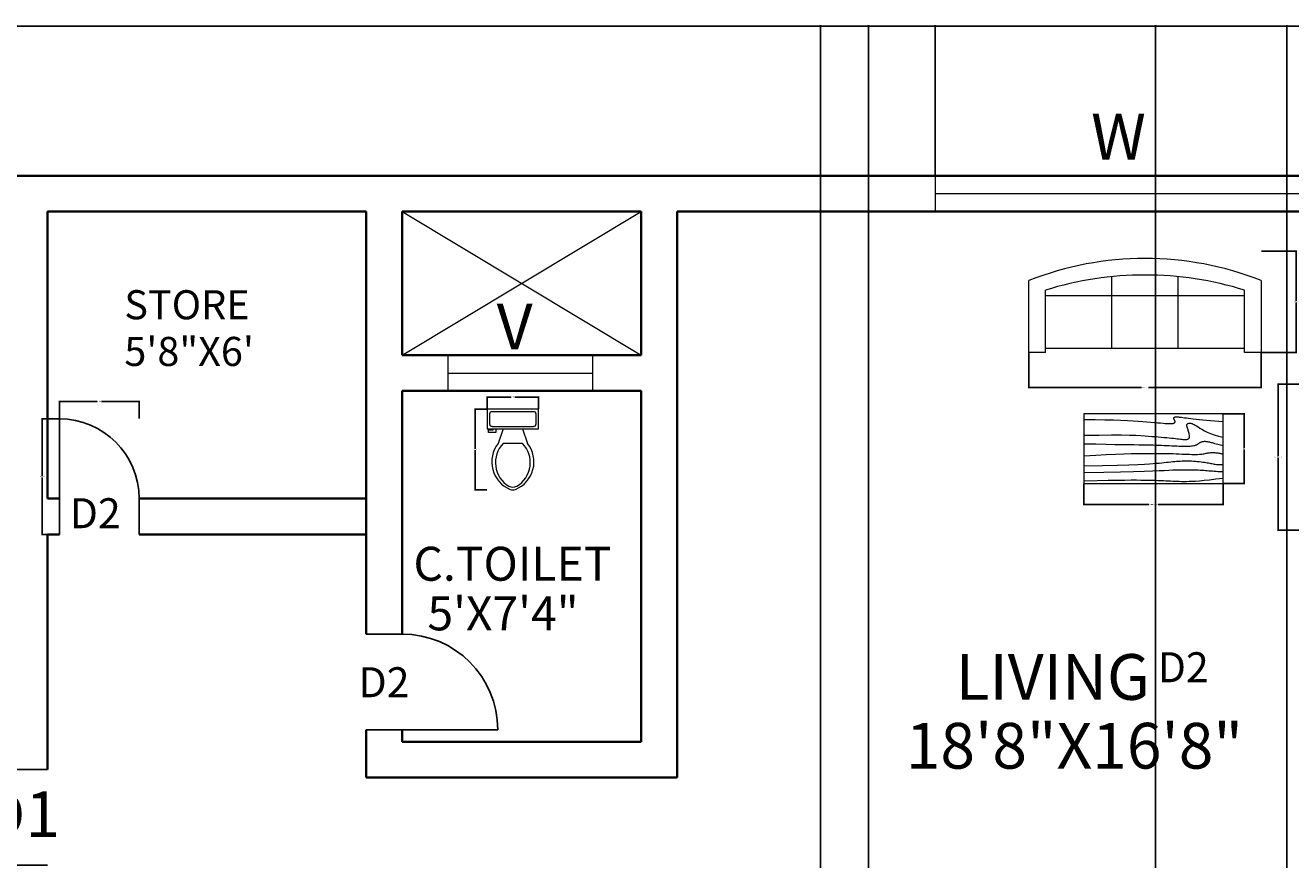
# Model space of a CAD drawing. Units: feet. Extents: x 1889 to 2708, y 1752 to 2375.
# Tile 4 of 5: x 2116 to 2434, y 2166 to 2375. Entities that reach past the tile are written whole.
import ezdxf

# ---------------------------------------------------------------- set-up
doc = ezdxf.new("R2010")
doc.units = ezdxf.units.FT
for name, color, linetype, lineweight in [('A-ANNO-DIMS', 2, 'Continuous', 18), ('A-ANNO-TEXT', 7, 'Continuous', 18), ('A-AREA-IDEN', 7, 'Continuous', 18), ('A-DOOR', 3, 'Continuous', 25), ('A-FLOR-FIXT', 8, 'Continuous', 18), ('A-FLOR-OPEN', 8, 'Continuous', 13), ('A-FURN', 8, 'Continuous', 18), ('A-GLAZ', 4, 'Continuous', 18), ('A-WALL', 7, 'Continuous', 35), ('C-PROP', 7, 'Continuous', 30)]:
    doc.layers.add(name, color=color, linetype=linetype, lineweight=lineweight)
doc.styles.get("Standard").update_dxf_attribs({"font": 'arial.ttf'})
doc.dimstyles.get("Standard").update_dxf_attribs({"dimtxt": 0.18, "dimasz": 0.18, "dimexe": 0.18, "dimexo": 0.0625, "dimgap": 0.09, "dimtad": 0, "dimtih": 1, "dimtoh": 1, "dimdec": 4, "dimzin": 0, "dimdsep": 46, "dimtxsty": 'Standard', "dimcen": 0.09, "dimadec": 0, "dimazin": 0, "dimtfac": 1, "dimtdec": 4, "dimtofl": 0, "dimtmove": 0, "dimatfit": 3, "dimfxl": 1, "dimtolj": 1, "dimtzin": 0, "dimarcsym": 0})

# ---------------------------------------------------------------- blocks, each defined once
blk = doc.blocks.new('Sofa - Roundback 7 ft.')
for p, q in [((-12.00002, -32.4421), (-12.00003, -6.5971)), ((11.99997, -32.4421), (11.99998, -6.5971)), ((-36.000027, -34), (-36.000027, -11.4696)), ((-35.999844, -13.3819), (35.9998, -13.3819)), ((35.99998, -34), (35.99998, -11.4696)), ((-36.000027, -32.4421), (35.99998, -32.4421))]:
    blk.add_line(p, q)
for points in [[(-36.000027, -34), (-42.000027, -34), (-42.000027, -8)], [(41.99998, -8), (41.99998, -34), (35.99998, -34)]]:
    blk.add_lwpolyline(points)
for centre, radius, start, end in [((0, -114.25), 114.25, 68.43141, 111.5686), ((-0.00001, -127.1968), 121.1968, 72.72033, 107.2797)]:
    blk.add_arc(centre, radius, start, end)
blk = doc.blocks.new('Table - Rectangular Woodgrain 60 x 30 in.')
for p, q in [((0, 0), (0, -30)), ((60, 0), (0, 0)), ((60, -30), (60, 0)), ((0, -30), (60, -30))]:
    blk.add_line(p, q)
for points in [[(0, -2.4), (4.8155, -2.418), (9.0302, -2.4688), (12.709, -2.5477), (15.9167, -2.65), (18.7181, -2.7711), (21.1781, -2.9063), (23.3616, -3.0508), (25.3333, -3.2), (27.1477, -3.3495), (28.8172, -3.4958), (30.3437, -3.636), (31.7291, -3.7667), (32.9756, -3.8849), (34.0849, -3.9875), (35.059, -4.0714), (35.9, -4.1334), (36.6114, -4.1711), (37.2041, -4.1854), (37.6906, -4.1779), (38.0833, -4.15), (38.3948, -4.1034), (38.6375, -4.0396), (38.8239, -3.9602), (38.9666, -3.8667), (39.0764, -3.7608), (39.1573, -3.6448), (39.2116, -3.521), (39.2416, -3.3917), (39.2498, -3.2593), (39.2385, -3.1261), (39.21, -2.9944), (39.1666, -2.8667), (39.111, -2.7447), (39.0468, -2.6281), (38.978, -2.5163), (38.9083, -2.4083), (38.8418, -2.3035), (38.7823, -2.201), (38.7337, -2.1001), (38.7, -2), (38.6844, -1.9003), (38.6875, -1.8021), (38.7094, -1.707), (38.75, -1.6167), (38.8094, -1.5326), (38.8875, -1.4563), (38.9844, -1.3893), (39.1, -1.3333), (39.2351, -1.2896), (39.3937, -1.2583), (39.5804, -1.2396), (39.8, -1.2333), (40.057, -1.2396), (40.3562, -1.2583), (40.7023, -1.2896), (41.1, -1.3333), (41.5547, -1.3895), (42.0755, -1.4573), (42.6721, -1.5361), (43.3542, -1.625), (44.1316, -1.7233), (45.014, -1.8302), (46.0114, -1.9449), (47.1333, -2.0667), (48.3862, -2.1947), (49.7625, -2.3281), (51.2513, -2.4663), (52.8416, -2.6083), (54.5226, -2.7535), (56.2833, -2.9011), (58.1127, -3.0501), (60, -3.2)], [(0, -9.2), (6.5759, -9.0858), (11.9385, -9.0365), (16.2527, -9.0418), (19.6833, -9.0917), (22.3952, -9.1759), (24.5531, -9.2844), (26.322, -9.4069), (27.8666, -9.5333), (29.3241, -9.6553), (30.7203, -9.7719), (32.0532, -9.8837), (33.3208, -9.9917), (34.5213, -10.0965), (35.6526, -10.199), (36.7128, -10.2999), (37.7, -10.4), (38.6129, -10.4996), (39.4531, -10.5969), (40.223, -10.6895), (40.925, -10.775), (41.5613, -10.8512), (42.1344, -10.9156), (42.6465, -10.966), (43.1, -11), (43.4976, -11.0158), (43.8437, -11.0136), (44.143, -10.9942), (44.4, -10.9583), (44.6195, -10.9069), (44.8062, -10.8406), (44.9648, -10.7603), (45.1, -10.6667), (45.2155, -10.5598), (45.3114, -10.4365), (45.3871, -10.2929), (45.4416, -10.125), (45.4743, -9.929), (45.4844, -9.7011), (45.4709, -9.4371), (45.4333, -9.1333), (45.3716, -8.7883), (45.2896, -8.4104), (45.1919, -8.0107), (45.0833, -7.6), (44.9685, -7.1893), (44.8521, -6.7896), (44.7388, -6.4117), (44.6333, -6.0667), (44.54, -5.7628), (44.4614, -5.4979), (44.4001, -5.2675), (44.3583, -5.0667), (44.3384, -4.8909), (44.3427, -4.7354), (44.3736, -4.5956), (44.4333, -4.4667), (44.5236, -4.3453), (44.6427, -4.2333), (44.7884, -4.1339), (44.9583, -4.05), (45.1501, -3.9849), (45.3614, -3.9417), (45.59, -3.9234), (45.8333, -3.9333), (46.0915, -3.9749), (46.3734, -4.0531), (46.6906, -4.1736), (47.0542, -4.3417), (47.4756, -4.5629), (47.9661, -4.8427), (48.5372, -5.1866), (49.2, -5.6), (49.9676, -6.0844), (50.8594, -6.625), (51.8965, -7.2031), (53.1, -7.8), (54.491, -8.3969), (56.0906, -8.975), (57.9199, -9.5156), (60, -10)], [(0, -12.8), (5.1847, -12.9322), (9.6213, -13.0323), (13.3963, -13.1059), (16.5958, -13.1583), (19.3063, -13.1952), (21.614, -13.2219), (23.6054, -13.2439), (25.3666, -13.2667), (26.9728, -13.2947), (28.4531, -13.3281), (29.8256, -13.3663), (31.1083, -13.4083), (32.3191, -13.4535), (33.476, -13.501), (34.597, -13.5501), (35.7, -13.6), (36.7984, -13.6497), (37.8875, -13.6979), (38.9578, -13.743), (40, -13.7833), (41.0047, -13.8174), (41.9625, -13.8438), (42.864, -13.8607), (43.7, -13.8667), (44.4631, -13.8604), (45.1552, -13.8417), (45.7801, -13.8104), (46.3416, -13.7667), (46.8439, -13.7104), (47.2906, -13.6417), (47.6858, -13.5604), (48.0333, -13.4667), (48.3375, -13.3608), (48.6042, -13.2448), (48.8396, -13.121), (49.05, -12.9917), (49.2417, -12.8593), (49.4208, -12.7261), (49.5937, -12.5944), (49.7667, -12.4667), (49.9452, -12.3451), (50.1323, -12.2313), (50.3303, -12.1268), (50.5416, -12.0333), (50.7686, -11.9524), (51.0135, -11.8854), (51.2788, -11.8341), (51.5666, -11.8), (51.8785, -11.7843), (52.2116, -11.7865), (52.562, -11.8059), (52.926, -11.8417), (53.2998, -11.8931), (53.6795, -11.9594), (54.0614, -12.0397), (54.4416, -12.1333), (54.8223, -12.2401), (55.2293, -12.3625), (55.6942, -12.5037), (56.2489, -12.6667), (56.9251, -12.8547), (57.7545, -13.0708), (58.7689, -13.3182), (60, -13.6)], [(0, -18), (5.124, -17.7273), (9.6609, -17.5057), (13.6705, -17.3303), (17.2125, -17.1958), (20.3467, -17.0973), (23.1328, -17.0297), (25.6307, -16.9878), (27.9, -16.9667), (29.9928, -16.9617), (31.9302, -16.9703), (33.7254, -16.9907), (35.3917, -17.0208), (36.9423, -17.0588), (38.3906, -17.1026), (39.7499, -17.1503), (41.0333, -17.2), (42.2519, -17.2496), (43.4073, -17.2969), (44.4986, -17.3395), (45.525, -17.375), (46.4858, -17.4012), (47.3802, -17.4156), (48.2074, -17.416), (48.9667, -17.4), (49.6583, -17.3662), (50.2872, -17.3167), (50.8595, -17.2547), (51.3812, -17.1833), (51.8584, -17.1057), (52.2971, -17.025), (52.7034, -16.9443), (53.0833, -16.8667), (53.443, -16.7951), (53.789, -16.7313), (54.128, -16.6768), (54.4666, -16.6334), (54.8115, -16.6024), (55.1693, -16.5854), (55.5465, -16.5841), (55.95, -16.6), (56.3828, -16.6337), (56.8346, -16.6823), (57.2915, -16.7418), (57.7396, -16.8084), (58.165, -16.878), (58.5539, -16.9469), (58.8924, -17.0111), (59.1666, -17.0667), (59.3679, -17.1107), (59.5078, -17.1438), (59.6032, -17.1675), (59.6708, -17.1833), (59.7275, -17.193), (59.7901, -17.1979), (59.8753, -17.1998), (60, -17.2)], [(0, -22.4), (8.0098, -22.2501), (14.4094, -22.1011), (19.4168, -21.9535), (23.25, -21.8083), (26.1269, -21.6663), (28.2656, -21.5281), (29.884, -21.3947), (31.2, -21.2667), (32.3967, -21.1448), (33.5172, -21.0292), (34.5697, -20.9198), (35.5625, -20.8167), (36.5037, -20.7198), (37.4015, -20.6292), (38.2642, -20.5448), (39.1, -20.4667), (39.9164, -20.3951), (40.7187, -20.3313), (41.5117, -20.2768), (42.3, -20.2333), (43.0883, -20.2024), (43.8812, -20.1854), (44.6836, -20.1841), (45.5, -20.2), (46.3328, -20.234), (47.1747, -20.2844), (48.0163, -20.3488), (48.8479, -20.425), (49.66, -20.5106), (50.4429, -20.6031), (51.1872, -20.7004), (51.8833, -20.8), (52.5246, -20.8999), (53.1166, -20.9995), (53.6681, -21.0983), (54.1875, -21.1958), (54.6834, -21.2919), (55.1646, -21.3859), (55.6394, -21.4777), (56.1167, -21.5667), (56.6028, -21.6515), (57.0961, -21.7266), (57.5929, -21.7852), (58.0896, -21.8208), (58.5823, -21.8268), (59.0674, -21.7964), (59.5412, -21.723), (60, -21.6)], [(0, -25.2), (8.6355, -25.0504), (15.7026, -24.9031), (21.4049, -24.7606), (25.9458, -24.625), (29.529, -24.4988), (32.3578, -24.3844), (34.6359, -24.284), (36.5667, -24.2), (38.3213, -24.1341), (39.9417, -24.0854), (41.437, -24.0523), (42.8167, -24.0333), (44.0901, -24.0268), (45.2667, -24.0313), (46.3557, -24.0451), (47.3667, -24.0667), (48.309, -24.0947), (49.1928, -24.1287), (50.0284, -24.168), (50.826, -24.2125), (51.5959, -24.2617), (52.3483, -24.3151), (53.0935, -24.3725), (53.8417, -24.4334), (54.6009, -24.497), (55.3699, -24.561), (56.1454, -24.6226), (56.9239, -24.6792), (57.7021, -24.7279), (58.4764, -24.7662), (59.2435, -24.7911), (60, -24.8)], [(0, -28.8), (5.6867, -28.6681), (10.45, -28.5698), (14.407, -28.5012), (17.675, -28.4584), (20.3711, -28.4374), (22.6125, -28.4344), (24.5164, -28.4455), (26.2, -28.4667), (27.762, -28.4947), (29.2276, -28.5281), (30.6033, -28.5663), (31.8958, -28.6084), (33.1118, -28.6535), (34.2578, -28.7011), (35.3405, -28.7501), (36.3666, -28.8), (37.3443, -28.8497), (38.288, -28.8974), (39.2137, -28.9412), (40.1375, -28.9792), (41.0753, -29.0093), (42.0432, -29.0297), (43.0572, -29.0384), (44.1333, -29.0333), (45.2936, -29.0114), (46.5843, -28.9641), (48.0579, -28.8816), (49.7666, -28.7542), (51.7629, -28.5721), (54.0989, -28.3255), (56.8272, -28.0048), (60, -27.6)]]:
    blk.add_lwpolyline(points)
blk = doc.blocks.new('Toilet - top')
for p, q in [((9.5, -6), (9.5, -2)), ((-10, -8.5), (-8, -8.5)), ((-10, -9.5), (-10, -8.5)), ((-7, -9.5), (-10, -9.5)), ((-8, -8.5), (-8, -8)), ((-7, -8), (-7, -9.5)), ((-4, -8), (-6, -14)), ((4, -8), (6, -14)), ((4, -14), (-4, -14))]:
    blk.add_line(p, q)
blk.add_lwpolyline([(10.5, -8), (10.5, 0), (-10.5, 0), (-10.5, -8)], close=True)
for points in [[(-9.5, -2), (-9.5, -6)], [(8.5, -1), (-8.5, -1)], [(-8.5, -7), (8.5, -7)]]:
    blk.add_lwpolyline(points)
for centre, radius, start, end in [((-8.62, -1.88), 0.884, 81.8699, 188.1301), ((8.62, -1.88), 0.884, 351.8699, 98.1301), ((-8.62, -6.12), 0.884, 171.8699, 278.1301), ((8.62, -6.12), 0.884, 261.8699, 8.1301), ((3.52, -21.58), 12.17, 141.4691, 247.9714), ((4.2, -21.82), 11.33, 136.3677, 238.9468), ((-3.52, -21.58), 12.17, 292.0284, 38.5307), ((-4.2, -21.82), 11.33, 301.053, 43.6321), ((0, -27.88), 4, 245.7318, 294.2682), ((0, -29), 4, 254.8605, 285.1395)]:
    blk.add_arc(centre, radius, start, end)
blk = doc.blocks.new('DOOR-SWING-24')
for p, q in [((9, 24), (0, 24)), ((33, 0), (0, 0))]:
    blk.add_line(p, q)
blk.add_arc((9, 0), 24, 0, 90)
blk = doc.blocks.new('DOOR-SWING-20')
for p, q in [((0, 29), (0, 0)), ((20, 9), (20, 0))]:
    blk.add_line(p, q)
blk.add_arc((0, 9), 20, 0, 90)
blk = doc.blocks.new('*D15')
at = {"layer": 'A-ANNO-DIMS', "color": 0, "lineweight": -2, "transparency": 16777216}
for p, q in [((2124.8, 2276.6), (2120.33, 2276.6)), ((2120.51, 2276.42), (2120.51, 2262.28)), ((2120.51, 2247.78), (2120.51, 2261.92)), ((2124.8, 2247.6), (2120.33, 2247.6))]:
    blk.add_line(p, q, dxfattribs=at)
at = {"layer": 'A-ANNO-DIMS', "color": 0, "transparency": 16777216}
for points in [[(2120.48, 2276.42), (2120.54, 2276.42), (2120.51, 2276.6)], [(2120.48, 2247.78), (2120.54, 2247.78), (2120.51, 2247.6)]]:
    blk.add_solid(points, dxfattribs=at)
at = {"layer": 'Defpoints', "color": 0, "transparency": 16777216}
for p in [(2120.51, 2276.6), (2124.86, 2276.6), (2124.86, 2247.6)]:
    blk.add_point(p, dxfattribs=at)
at = {"layer": 'A-ANNO-DIMS', "color": 0, "transparency": 16777216, "insert": (2120.51, 2262.1), "char_height": 0.18, "attachment_point": 5}
blk.add_mtext('\\A1;DOOR 29 TYP.', dxfattribs=at)
blk = doc.blocks.new('*D16')
at = {"layer": 'A-ANNO-DIMS', "color": 0, "lineweight": -2, "transparency": 16777216}
for p, q in [((2124.86, 2276.66), (2124.86, 2281.13)), ((2125.04, 2280.95), (2134.33, 2280.95)), ((2144.68, 2280.95), (2135.39, 2280.95)), ((2144.86, 2276.66), (2144.86, 2281.13))]:
    blk.add_line(p, q, dxfattribs=at)
at = {"layer": 'A-ANNO-DIMS', "color": 0, "transparency": 16777216}
for points in [[(2125.04, 2280.98), (2125.04, 2280.92), (2124.86, 2280.95)], [(2144.68, 2280.98), (2144.68, 2280.92), (2144.86, 2280.95)]]:
    blk.add_solid(points, dxfattribs=at)
at = {"layer": 'Defpoints', "color": 0, "transparency": 16777216}
for p in [(2144.86, 2280.95), (2124.86, 2276.6), (2144.86, 2276.6)]:
    blk.add_point(p, dxfattribs=at)
at = {"layer": 'A-ANNO-DIMS', "color": 0, "transparency": 16777216, "insert": (2134.86, 2280.95), "char_height": 0.18, "attachment_point": 5}
blk.add_mtext('\\A1;20 TYP.', dxfattribs=at)
blk = doc.blocks.new('*D17')
at = {"layer": 'A-ANNO-DIMS', "color": 0, "lineweight": -2, "transparency": 16777216}
for p, q in [((2232.14, 2279.01), (2228.98, 2279.01)), ((2229.16, 2278.83), (2229.16, 2269.07)), ((2229.16, 2258.94), (2229.16, 2268.7)), ((2232.14, 2258.76), (2228.98, 2258.76))]:
    blk.add_line(p, q, dxfattribs=at)
at = {"layer": 'A-ANNO-DIMS', "color": 0, "transparency": 16777216}
for points in [[(2229.13, 2278.83), (2229.19, 2278.83), (2229.16, 2279.01)], [(2229.13, 2258.94), (2229.19, 2258.94), (2229.16, 2258.76)]]:
    blk.add_solid(points, dxfattribs=at)
at = {"layer": 'Defpoints', "color": 0, "transparency": 16777216}
for p in [(2229.16, 2279.01), (2232.2, 2279.01), (2232.2, 2258.76)]:
    blk.add_point(p, dxfattribs=at)
at = {"layer": 'A-ANNO-DIMS', "color": 0, "transparency": 16777216, "insert": (2229.16, 2268.88), "char_height": 0.18, "attachment_point": 5}
blk.add_mtext('\\A1;WC 20 TYP.', dxfattribs=at)
blk = doc.blocks.new('*D18')
at = {"layer": 'A-ANNO-DIMS', "color": 0, "lineweight": -2, "transparency": 16777216}
for p, q in [((2232.2, 2279.07), (2232.2, 2282.22)), ((2232.38, 2282.04), (2238.11, 2282.04)), ((2244.88, 2282.04), (2239.15, 2282.04)), ((2245.06, 2279.07), (2245.06, 2282.22))]:
    blk.add_line(p, q, dxfattribs=at)
at = {"layer": 'A-ANNO-DIMS', "color": 0, "transparency": 16777216}
for points in [[(2232.38, 2282.07), (2232.38, 2282.01), (2232.2, 2282.04)], [(2244.88, 2282.07), (2244.88, 2282.01), (2245.06, 2282.04)]]:
    blk.add_solid(points, dxfattribs=at)
at = {"layer": 'Defpoints', "color": 0, "transparency": 16777216}
for p in [(2245.06, 2282.04), (2232.2, 2279.01), (2245.06, 2279.01)]:
    blk.add_point(p, dxfattribs=at)
at = {"layer": 'A-ANNO-DIMS', "color": 0, "transparency": 16777216, "insert": (2238.63, 2282.04), "char_height": 0.18, "attachment_point": 5}
blk.add_mtext('\\A1;13 TYP.', dxfattribs=at)
blk = doc.blocks.new('*D23')
at = {"layer": 'A-ANNO-DIMS', "color": 0, "lineweight": -2, "transparency": 16777216}
for p, q in [((2368.1, 2293.18), (2368.1, 2284.32)), ((2426.4, 2293.18), (2426.4, 2284.32)), ((2368.28, 2284.5), (2396.35, 2284.5)), ((2426.22, 2284.5), (2398.16, 2284.5))]:
    blk.add_line(p, q, dxfattribs=at)
at = {"layer": 'A-ANNO-DIMS', "color": 0, "transparency": 16777216}
for points in [[(2368.28, 2284.53), (2368.28, 2284.47), (2368.1, 2284.5)], [(2426.22, 2284.53), (2426.22, 2284.47), (2426.4, 2284.5)]]:
    blk.add_solid(points, dxfattribs=at)
at = {"layer": 'Defpoints', "color": 0, "transparency": 16777216}
for p in [(2368.1, 2293.24), (2426.4, 2293.24), (2426.4, 2284.5)]:
    blk.add_point(p, dxfattribs=at)
at = {"layer": 'A-ANNO-DIMS', "color": 0, "transparency": 16777216, "insert": (2397.25, 2284.5), "char_height": 0.18, "attachment_point": 5}
blk.add_mtext('\\A1;SOFA 58 TYP.', dxfattribs=at)
blk = doc.blocks.new('*D24')
at = {"layer": 'A-ANNO-DIMS', "color": 0, "lineweight": -2, "transparency": 16777216}
for p, q in [((2426.47, 2318.69), (2435.33, 2318.69)), ((2435.15, 2318.51), (2435.15, 2306.15)), ((2435.15, 2293.42), (2435.15, 2305.78)), ((2426.47, 2293.24), (2435.33, 2293.24))]:
    blk.add_line(p, q, dxfattribs=at)
at = {"layer": 'A-ANNO-DIMS', "color": 0, "transparency": 16777216}
for points in [[(2435.12, 2318.51), (2435.18, 2318.51), (2435.15, 2318.69)], [(2435.12, 2293.42), (2435.18, 2293.42), (2435.15, 2293.24)]]:
    blk.add_solid(points, dxfattribs=at)
at = {"layer": 'Defpoints', "color": 0, "transparency": 16777216}
for p in [(2426.4, 2318.69), (2435.15, 2318.69), (2426.4, 2293.24)]:
    blk.add_point(p, dxfattribs=at)
at = {"layer": 'A-ANNO-DIMS', "color": 0, "transparency": 16777216, "insert": (2435.15, 2305.97), "char_height": 0.18, "attachment_point": 5}
blk.add_mtext('\\A1;25 TYP.', dxfattribs=at)
blk = doc.blocks.new('*D25')
at = {"layer": 'A-ANNO-DIMS', "color": 0, "lineweight": -2, "transparency": 16777216}
for p, q in [((2436.07, 2285.32), (2430.47, 2285.32)), ((2430.65, 2285.14), (2430.65, 2267.2)), ((2430.65, 2248.89), (2430.65, 2266.83)), ((2436.07, 2248.71), (2430.47, 2248.71))]:
    blk.add_line(p, q, dxfattribs=at)
at = {"layer": 'A-ANNO-DIMS', "color": 0, "transparency": 16777216}
for points in [[(2430.62, 2285.14), (2430.68, 2285.14), (2430.65, 2285.32)], [(2430.62, 2248.89), (2430.68, 2248.89), (2430.65, 2248.71)]]:
    blk.add_solid(points, dxfattribs=at)
at = {"layer": 'Defpoints', "color": 0, "transparency": 16777216}
for p in [(2436.14, 2285.32), (2430.65, 2248.71), (2436.14, 2248.71)]:
    blk.add_point(p, dxfattribs=at)
at = {"layer": 'A-ANNO-DIMS', "color": 0, "transparency": 16777216, "insert": (2430.65, 2267.01), "char_height": 0.18, "attachment_point": 5}
blk.add_mtext('\\A1;LOVESEAT 37 TYP.', dxfattribs=at)
blk = doc.blocks.new('*D29')
at = {"layer": 'A-ANNO-DIMS', "color": 0, "lineweight": -2, "transparency": 16777216}
for p, q in [((2381.91, 2260.29), (2381.91, 2254.93)), ((2416.86, 2260.29), (2416.86, 2254.93)), ((2382.09, 2255.11), (2398.19, 2255.11)), ((2416.68, 2255.11), (2400.58, 2255.11))]:
    blk.add_line(p, q, dxfattribs=at)
at = {"layer": 'A-ANNO-DIMS', "color": 0, "transparency": 16777216}
for points in [[(2382.09, 2255.14), (2382.09, 2255.08), (2381.91, 2255.11)], [(2416.68, 2255.14), (2416.68, 2255.08), (2416.86, 2255.11)]]:
    blk.add_solid(points, dxfattribs=at)
at = {"layer": 'Defpoints', "color": 0, "transparency": 16777216}
for p in [(2381.91, 2260.35), (2416.86, 2260.35), (2416.86, 2255.11)]:
    blk.add_point(p, dxfattribs=at)
at = {"layer": 'A-ANNO-DIMS', "color": 0, "transparency": 16777216, "insert": (2399.38, 2255.11), "char_height": 0.18, "attachment_point": 5}
blk.add_mtext('\\A1;COFFEE TABLE 35', dxfattribs=at)
blk = doc.blocks.new('*D30')
at = {"layer": 'A-ANNO-DIMS', "color": 0, "lineweight": -2, "transparency": 16777216}
for p, q in [((2416.93, 2277.83), (2422.29, 2277.83)), ((2422.11, 2277.65), (2422.11, 2269.27)), ((2422.11, 2260.53), (2422.11, 2268.91)), ((2416.93, 2260.35), (2422.29, 2260.35))]:
    blk.add_line(p, q, dxfattribs=at)
at = {"layer": 'A-ANNO-DIMS', "color": 0, "transparency": 16777216}
for points in [[(2422.08, 2277.65), (2422.14, 2277.65), (2422.11, 2277.83)], [(2422.08, 2260.53), (2422.14, 2260.53), (2422.11, 2260.35)]]:
    blk.add_solid(points, dxfattribs=at)
at = {"layer": 'Defpoints', "color": 0, "transparency": 16777216}
for p in [(2416.86, 2277.83), (2422.11, 2277.83), (2416.86, 2260.35)]:
    blk.add_point(p, dxfattribs=at)
at = {"layer": 'A-ANNO-DIMS', "color": 0, "transparency": 16777216, "insert": (2422.11, 2269.09), "char_height": 0.18, "attachment_point": 5}
blk.add_mtext('\\A1;17', dxfattribs=at)
blk = doc.blocks.new('*D38')
at = {"layer": 'A-ANNO-DIMS', "color": 0, "lineweight": -2, "transparency": 16777216}
for p, q in [((2082.41, 2337.66), (2082.41, 2375.33)), ((2082.59, 2375.15), (2213.05, 2375.15)), ((2344.45, 2375.15), (2213.98, 2375.15)), ((2344.63, 2337.66), (2344.63, 2375.33))]:
    blk.add_line(p, q, dxfattribs=at)
at = {"layer": 'A-ANNO-DIMS', "color": 0, "transparency": 16777216}
for points in [[(2082.59, 2375.18), (2082.59, 2375.12), (2082.41, 2375.15)], [(2344.45, 2375.18), (2344.45, 2375.12), (2344.63, 2375.15)]]:
    blk.add_solid(points, dxfattribs=at)
at = {"layer": 'Defpoints', "color": 0, "transparency": 16777216}
for p in [(2344.63, 2375.15), (2082.41, 2337.6), (2344.63, 2337.6)]:
    blk.add_point(p, dxfattribs=at)
at = {"layer": 'A-ANNO-DIMS', "color": 0, "transparency": 16777216, "insert": (2213.52, 2375.15), "char_height": 0.18, "attachment_point": 5}
blk.add_mtext('\\A1;262.23', dxfattribs=at)
blk = doc.blocks.new('*D39')
at = {"layer": 'A-ANNO-DIMS', "color": 0, "lineweight": -2, "transparency": 16777216}
for p, q in [((2344.63, 2337.66), (2344.63, 2375.33)), ((2344.81, 2375.15), (2395.36, 2375.15)), ((2446.46, 2375.15), (2395.92, 2375.15)), ((2446.64, 2337.66), (2446.64, 2375.33))]:
    blk.add_line(p, q, dxfattribs=at)
at = {"layer": 'A-ANNO-DIMS', "color": 0, "transparency": 16777216}
for points in [[(2344.81, 2375.18), (2344.81, 2375.12), (2344.63, 2375.15)], [(2446.46, 2375.18), (2446.46, 2375.12), (2446.64, 2375.15)]]:
    blk.add_solid(points, dxfattribs=at)
at = {"layer": 'Defpoints', "color": 0, "transparency": 16777216}
for p in [(2446.64, 2375.15), (2344.63, 2337.6), (2446.64, 2337.6)]:
    blk.add_point(p, dxfattribs=at)
at = {"layer": 'A-ANNO-DIMS', "color": 0, "transparency": 16777216, "insert": (2395.64, 2375.15), "char_height": 0.18, "attachment_point": 5}
blk.add_mtext('\\A1;102', dxfattribs=at)
blk = doc.blocks.new('*D48')
at = {"layer": 'A-ANNO-DIMS', "color": 0, "lineweight": -2, "transparency": 16777216}
for p, q in [((1983.86, 1820.66), (1983.86, 2375.33)), ((1984.04, 2375.15), (2208.07, 2375.15)), ((2432.68, 2375.15), (2208.66, 2375.15)), ((2432.86, 1820.66), (2432.86, 2375.33))]:
    blk.add_line(p, q, dxfattribs=at)
at = {"layer": 'A-ANNO-DIMS', "color": 0, "transparency": 16777216}
for points in [[(1984.04, 2375.18), (1984.04, 2375.12), (1983.86, 2375.15)], [(2432.68, 2375.18), (2432.68, 2375.12), (2432.86, 2375.15)]]:
    blk.add_solid(points, dxfattribs=at)
at = {"layer": 'Defpoints', "color": 0, "transparency": 16777216}
for p in [(2432.86, 2375.15), (1983.86, 1820.6), (2432.86, 1820.6)]:
    blk.add_point(p, dxfattribs=at)
at = {"layer": 'A-ANNO-DIMS', "color": 0, "transparency": 16777216, "insert": (2208.36, 2375.15), "char_height": 0.18, "attachment_point": 5}
blk.add_mtext('\\A1;449', dxfattribs=at)
blk = doc.blocks.new('*D61')
at = {"layer": 'A-ANNO-DIMS', "color": 0, "lineweight": -2, "transparency": 16777216}
for p, q in [((2315.86, 1909.16), (2315.86, 2375.33)), ((2316.04, 2375.15), (2321.65, 2375.15)), ((2327.68, 2375.15), (2322.07, 2375.15)), ((2327.86, 1913.66), (2327.86, 2375.33))]:
    blk.add_line(p, q, dxfattribs=at)
at = {"layer": 'A-ANNO-DIMS', "color": 0, "transparency": 16777216}
for points in [[(2316.04, 2375.18), (2316.04, 2375.12), (2315.86, 2375.15)], [(2327.68, 2375.18), (2327.68, 2375.12), (2327.86, 2375.15)]]:
    blk.add_solid(points, dxfattribs=at)
at = {"layer": 'Defpoints', "color": 0, "transparency": 16777216}
for p in [(2327.86, 2375.15), (2327.86, 1913.6), (2315.86, 1909.1)]:
    blk.add_point(p, dxfattribs=at)
at = {"layer": 'A-ANNO-DIMS', "color": 0, "transparency": 16777216, "insert": (2321.86, 2375.15), "char_height": 0.18, "attachment_point": 5}
blk.add_mtext('\\A1;12', dxfattribs=at)
blk = doc.blocks.new('*D64')
at = {"layer": 'A-ANNO-DIMS', "color": 0, "lineweight": -2, "transparency": 16777216}
for p, q in [((2327.86, 2011.66), (2327.86, 2375.33)), ((2328.04, 2375.15), (2363.65, 2375.15)), ((2399.68, 2375.15), (2364.08, 2375.15)), ((2399.86, 2011.66), (2399.86, 2375.33))]:
    blk.add_line(p, q, dxfattribs=at)
at = {"layer": 'A-ANNO-DIMS', "color": 0, "transparency": 16777216}
for points in [[(2328.04, 2375.18), (2328.04, 2375.12), (2327.86, 2375.15)], [(2399.68, 2375.18), (2399.68, 2375.12), (2399.86, 2375.15)]]:
    blk.add_solid(points, dxfattribs=at)
at = {"layer": 'Defpoints', "color": 0, "transparency": 16777216}
for p in [(2399.86, 2375.15), (2327.86, 2011.6), (2399.86, 2011.6)]:
    blk.add_point(p, dxfattribs=at)
at = {"layer": 'A-ANNO-DIMS', "color": 0, "transparency": 16777216, "insert": (2363.86, 2375.15), "char_height": 0.18, "attachment_point": 5}
blk.add_mtext('\\A1;72', dxfattribs=at)

msp = doc.modelspace()

# ---------------------------------------------------------------- linework, layer by layer
at = {"layer": 'A-FLOR-OPEN'}
for p, q in [((2210.8644, 2328.5988), (2270.8644, 2292.5988)), ((2210.8644, 2292.5988), (2270.8644, 2328.5988))]:
    msp.add_line(p, q, dxfattribs=at)
at = {"layer": 'A-GLAZ'}
for p, q in [((2344.6329, 2337.5988), (2344.6329, 2328.5988)), ((2344.6329, 2333.0988), (2446.6414, 2333.0988)), ((2222.3553, 2292.5988), (2222.3553, 2283.5988)), ((2258.6501, 2292.5988), (2258.6501, 2283.5988)), ((2222.3553, 2288.0988), (2258.6501, 2288.0988))]:
    msp.add_line(p, q, dxfattribs=at)
at = {"layer": 'A-WALL'}
for p, q in [((1992.8644, 2337.5988), (2669.8644, 2337.5988)), ((2121.8644, 2337.5988), (2201.8644, 2337.5988)), ((2210.8644, 2337.5988), (2270.8644, 2337.5988)), ((2279.8644, 2337.5988), (2503.8644, 2337.5988)), ((2121.8644, 2328.5988), (2121.8644, 2256.5988)), ((2121.8644, 2328.5988), (2201.8644, 2328.5988)), ((2201.8644, 2328.5988), (2201.8644, 2256.5988)), ((2210.8644, 2328.5988), (2210.8644, 2292.5988)), ((2210.8644, 2328.5988), (2270.8644, 2328.5988)), ((2270.8644, 2328.5988), (2270.8644, 2292.5988)), ((2279.8644, 2328.5988), (2279.8644, 2186.5988)), ((2279.8644, 2328.5988), (2503.8644, 2328.5988)), ((2270.8644, 2292.5988), (2210.8644, 2292.5988)), ((2270.8644, 2283.5988), (2210.8644, 2283.5988)), ((2210.8644, 2283.5988), (2210.8644, 2256.5988)), ((2270.8644, 2283.5988), (2270.8644, 2195.5988)), ((2279.8644, 2283.5988), (2279.8644, 2195.5988)), ((2124.8644, 2256.5988), (2121.8644, 2256.5988)), ((2201.8644, 2256.5988), (2144.8644, 2256.5988)), ((2201.8644, 2222.5988), (2201.8644, 2256.5988)), ((2210.8644, 2222.5988), (2210.8644, 2256.5988)), ((2121.8644, 2247.5988), (2121.8644, 2188.5988)), ((2124.8644, 2247.5988), (2121.8644, 2247.5988)), ((2201.8644, 2247.5988), (2144.8644, 2247.5988)), ((2201.8644, 2186.5988), (2201.8644, 2198.5988)), ((2210.8644, 2195.5988), (2210.8644, 2198.5988)), ((2270.8644, 2195.5988), (2210.8644, 2195.5988)), ((2279.8644, 2186.5988), (2279.8644, 2195.5988)), ((2121.8644, 2188.5988), (2121.8644, 2191.5988)), ((2279.8644, 2186.5988), (2201.8644, 2186.5988))]:
    msp.add_line(p, q, dxfattribs=at)
at = {"layer": 'C-PROP'}
msp.add_line((1926.8644, 2337.5988), (2669.8644, 2337.5988), dxfattribs=at)

# ---------------------------------------------------------------- block references
at = {"layer": 'A-DOOR'}
for name, p in [('DOOR-SWING-20', (2124.864, 2247.599)), ('DOOR-SWING-24', (2201.864, 2198.599))]:
    msp.add_blockref(name, p, dxfattribs=at)
at = {"layer": 'A-DOOR', "rotation": 180}
msp.add_blockref('DOOR-SWING-24', (2121.8649, 2188.5986), dxfattribs=at)
at = {"layer": 'A-FLOR-FIXT', "xscale": 0.6125984407344605, "yscale": 0.6125984407344605, "zscale": 0.6125984407344605}
msp.add_blockref('Toilet - top', (2238.6315, 2279.0069), dxfattribs=at)
at = {"layer": 'A-FURN'}
for name, p, xscale, yscale, zscale in [('Sofa - Roundback 7 ft.', (2397.2514, 2316.8411), 0.694114071376089, 0.694114071376089, 0.694114071376089), ('Table - Rectangular Woodgrain 60 x 30 in.', (2381.9055, 2277.8277), 0.5826300696864751, 0.5826300696864751, 0.5826300696864751)]:
    msp.add_blockref(name, p, dxfattribs=dict(at, xscale=xscale, yscale=yscale, zscale=zscale))

# ---------------------------------------------------------------- texts
at = {"layer": 'A-ANNO-TEXT'}
for s, height, p in [('W', 11.4692, (2383.7224, 2341.6557)), ('V', 11.4692, (2234.5884, 2294.0043)), ('D2', 7.52883, (2127.4747, 2249.1529)), ('D2', 7.52883, (2400.4549, 2210.5078)), ('D2', 7.52883, (2199.926, 2206.7465)), ('D1', 11.46921, (2105.5594, 2171.6646))]:
    msp.add_text(s, height=height, dxfattribs=at).set_placement(p)
at = {"layer": 'A-AREA-IDEN'}
for s, height, p in [('STORE', 7.29353, (2141.1503, 2301.5767)), ('5\'8"X6\'', 7.29353, (2141.1503, 2289.8603)), ('C.TOILET', 8.50697, (2213.6906, 2235.9899)), ('5\'X7\'4"', 8.50697, (2217.2073, 2223.5359)), ('LIVING', 11.46921, (2349.7242, 2206.1071)), ('18\'8"X16\'8"', 11.469207, (2337.2218, 2188.8539))]:
    msp.add_text(s, height=height, dxfattribs=at).set_placement(p)

# ---------------------------------------------------------------- dimensions: what is measured, and where the dimension line sits
at = {"layer": 'A-ANNO-DIMS'}
for base, p1, p2, override, picture, middle in [((2432.8644, 2375.1488), (1983.8644, 1820.5988), (2432.8644, 1820.5988), {"dimdec": 0, "dimlfac": 1, "dimrnd": 0, "dimzin": 0, "dimdsep": 46, "dimlunit": 2}, '*D48', (2208.3644, 2375.1488)), ((2344.6329, 2375.1488), (2082.4064, 2337.5988), (2344.6329, 2337.5988), {"dimdec": 2, "dimlfac": 1, "dimrnd": 0, "dimzin": 0, "dimdsep": 46, "dimlunit": 2}, '*D38', (2213.5196, 2375.1488)), ((2327.8644, 2375.1488), (2315.8644, 1909.0988), (2327.8644, 1913.5988), {"dimdec": 0, "dimlfac": 1, "dimrnd": 0, "dimzin": 0, "dimdsep": 46, "dimlunit": 2}, '*D61', (2321.8644, 2375.1488)), ((2399.8644, 2375.1488), (2327.8644, 2011.5988), (2399.8644, 2011.5988), {"dimdec": 0, "dimlfac": 1, "dimrnd": 0, "dimzin": 0, "dimdsep": 46, "dimlunit": 2}, '*D64', (2363.8644, 2375.1488)), ((2446.6414, 2375.1488), (2344.6329, 2337.5988), (2446.6414, 2337.5988), {"dimdec": 0, "dimlfac": 1, "dimrnd": 0, "dimzin": 0, "dimdsep": 46, "dimlunit": 2}, '*D39', (2395.6371, 2375.1488))]:
    dim = msp.add_linear_dim(base=base, p1=p1, p2=p2, dimstyle='Standard', override=override, dxfattribs=at)
    dim.commit()
    dim.dimension.update_dxf_attribs({"geometry": picture, "text_midpoint": middle})
for base, p1, p2, angle, text, picture, middle in [((2435.15, 2318.6921), (2426.4042, 2293.2413), (2426.4042, 2318.6921), 90, '<> TYP.', '*D24', (2435.15, 2305.9667)), ((2430.6453, 2248.7132), (2436.1357, 2285.3157), (2436.1357, 2248.7132), 270, 'LOVESEAT <> TYP.', '*D25', (2430.6453, 2267.0144)), ((2120.5144, 2276.5988), (2124.8644, 2247.5988), (2124.8644, 2276.5988), 90, 'DOOR <> TYP.', '*D15', (2120.5144, 2262.0988)), ((2229.1626, 2279.0069), (2232.1992, 2258.7628), (2232.1992, 2279.0069), 90, 'WC <> TYP.', '*D17', (2229.1626, 2268.8848))]:
    dim = msp.add_linear_dim(base=base, p1=p1, p2=p2, angle=angle, text=text, dimstyle='Standard', override={"dimdec": 0, "dimlfac": 1, "dimrnd": 0, "dimzin": 0, "dimdsep": 46, "dimlunit": 2}, dxfattribs=at)
    dim.commit()
    dim.dimension.update_dxf_attribs({"geometry": picture, "text_midpoint": middle})
for base, p1, p2, text, picture, middle in [((2426.4042, 2284.4954), (2368.0986, 2293.2413), (2426.4042, 2293.2413), 'SOFA <> TYP.', '*D23', (2397.2514, 2284.4954)), ((2144.8644, 2280.9488), (2124.8644, 2276.5988), (2144.8644, 2276.5988), '<> TYP.', '*D16', (2134.8644, 2280.9488)), ((2245.0637, 2282.0435), (2232.1992, 2279.0069), (2245.0637, 2279.0069), '<> TYP.', '*D18', (2238.6315, 2282.0435)), ((2416.8633, 2255.1052), (2381.9055, 2260.3488), (2416.8633, 2260.3488), 'COFFEE TABLE <>', '*D29', (2399.3844, 2255.1052))]:
    dim = msp.add_linear_dim(base=base, p1=p1, p2=p2, text=text, dimstyle='Standard', override={"dimdec": 0, "dimlfac": 1, "dimrnd": 0, "dimzin": 0, "dimdsep": 46, "dimlunit": 2}, dxfattribs=at)
    dim.commit()
    dim.dimension.update_dxf_attribs({"geometry": picture, "text_midpoint": middle})
dim = msp.add_linear_dim(base=(2422.107, 2277.8277), p1=(2416.8633, 2260.3488), p2=(2416.8633, 2277.8277), angle=90, dimstyle='Standard', override={"dimdec": 0, "dimlfac": 1, "dimrnd": 0, "dimzin": 0, "dimdsep": 46, "dimlunit": 2}, dxfattribs=at)
dim.commit()
dim.dimension.update_dxf_attribs({"geometry": '*D30', "text_midpoint": (2422.107, 2269.0883)})

doc.saveas('drawing.dxf')
